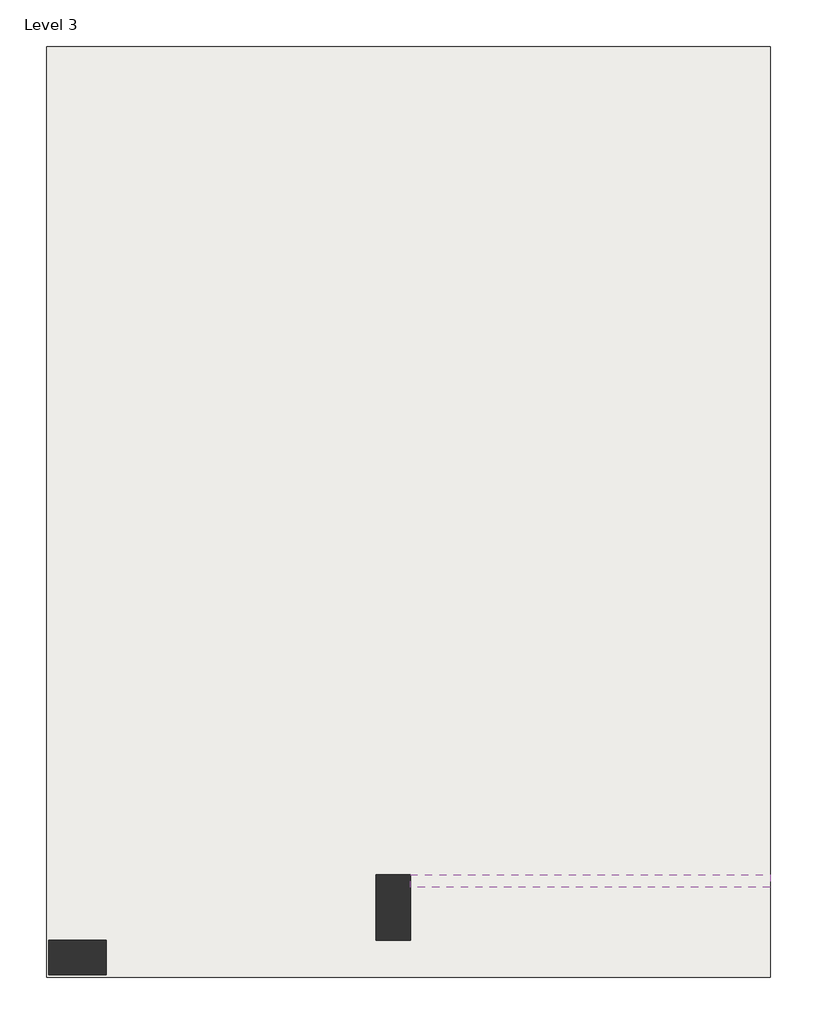
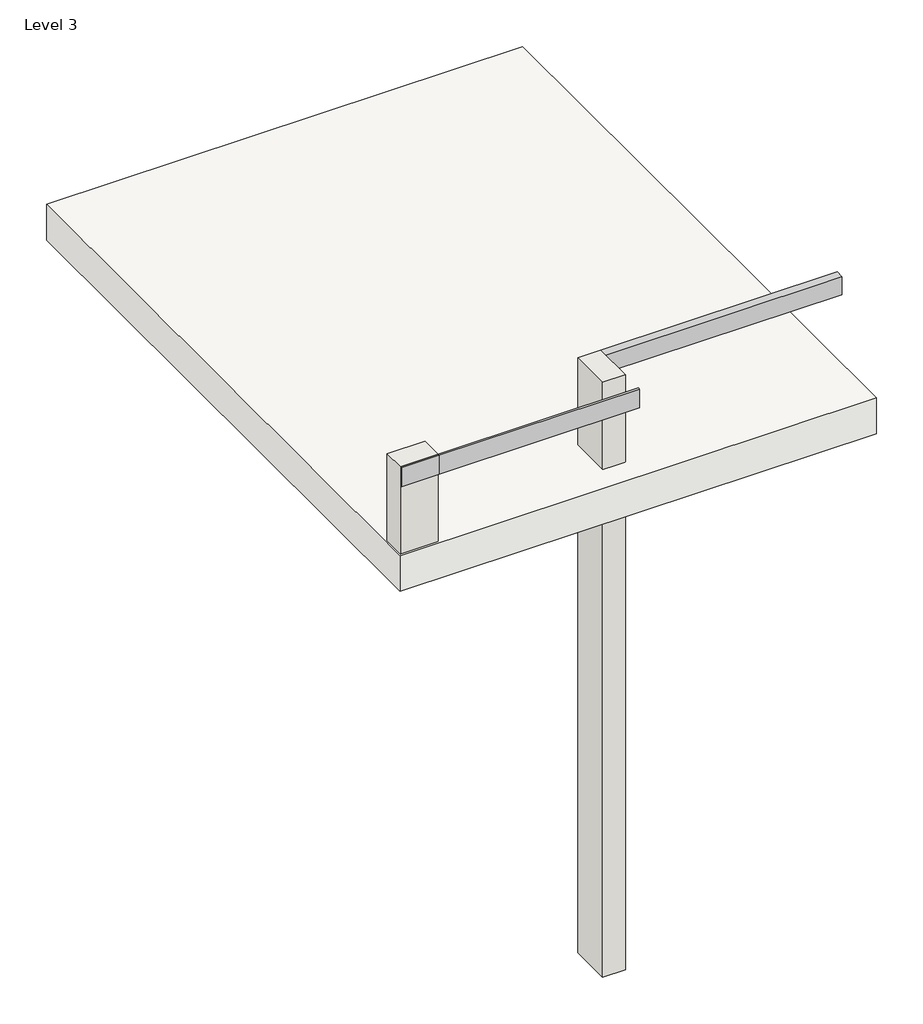
# One storey: 2 walls, 1 proxy, 1 roof.
"""IFC4 building model written with IfcOpenShell, lengths in millimetres."""

from ifc_helpers import new_model, si_unit, frame, origin, place, context, project, spatial, polyline, outline, extrude, faceted_brep, transform, mapped, element, save
from components import generic_models_1_generic_models_1_5385a8bd

model = new_model("IFC4")

# Units and contexts
model_context = context("Model", 3, world=origin())
ifc_project = project(units=[si_unit("LENGTHUNIT", "METRE", prefix="MILLI")], contexts=[model_context])

# Site, building, storey
site = spatial("IfcSite", under=ifc_project)
building = spatial("IfcBuilding", under=site)
storey = spatial("IfcBuildingStorey", under=building, Name="Level 3", Elevation=6705.6)

# Proxy
placement = place(None, origin())
generic_models_1_generic_models_1_shape = generic_models_1_generic_models_1_5385a8bd(model_context)
element("IfcBuildingElementProxy", 1, Name="Generic Models 1 : Generic Models 1", ObjectType="Generic Models 1 : Generic Models 1", at=placement, inside=storey, context=model_context, shape_type="MappedRepresentation", body=[
    mapped(generic_models_1_generic_models_1_shape, transform((0.0, 0.0, 0.0), x_axis=(1.0, 0.0, 0.0), y_axis=(0.0, 1.0, 0.0), z_axis=(0.0, 0.0, 1.0))),
])

# Roof
element("IfcRoof", 2, ObjectType="Generic - 18\"", at=placement, inside=storey, context=model_context, shape_type="SweptSolid", body=[
    extrude(outline(polyline([(-13364.9465329, 11213.7598519), (-6964.1465329, 11213.7598519), (-6964.1465329, 2984.1598519), (-13364.9465329, 2984.1598519), (-13364.9465329, 11213.7598519)])), frame((0.0, 0.0, 6705.6), z_axis=(0.0, 0.0, 1.0), x_axis=(1.0, 0.0, 0.0)), (0.0, 0.0, 1.0), 508.0),
])

# Walls
element("IfcWall", 3, ObjectType="Generic - 12\"", at=placement, inside=storey, context=model_context, shape_type="Brep", body=[
    faceted_brep([(-12837.2306534, 3314.3598519, 6705.6), (-13345.2306534, 3314.3598519, 6705.6), (-13345.2306534, 3314.3598519, 7213.6), (-13345.2306534, 3314.3598519, 8451.8321088), (-12837.2306534, 3314.3598519, 8451.8321088), (-12837.2306534, 3314.3598519, 7213.6), (-12837.2306534, 3009.5598519, 6705.6), (-12837.2306534, 3009.5598519, 8451.8321088), (-13345.2306534, 3009.5598519, 8451.8321088), (-13345.2306534, 3009.5598519, 6705.6)], [[[0, 1, 2, 3, 4, 5]], [[6, 7, 8, 9]], [[1, 0, 6, 9]], [[3, 2, 1, 9, 8]], [[4, 3, 8, 7]], [[0, 5, 4, 7, 6]]]),
])
element("IfcWall", 4, ObjectType="Generic - 12\"", at=placement, inside=storey, context=model_context, shape_type="Brep", body=[
    faceted_brep([(-10144.8306534, 3314.3598519, 0.0), (-10144.8306534, 3890.6797737, 0.0), (-10144.8306534, 3890.6797737, 8451.8321088), (-10144.8306534, 3314.3598519, 8451.8321088), (-10144.8306534, 3314.3598519, 3048.0), (-10449.6306534, 3314.3598519, 0.0), (-10449.6306534, 3314.3598519, 8451.8321088), (-10449.6306534, 3890.6797737, 8451.8321088), (-10449.6306534, 3890.6797737, 8396.4882518), (-10449.6306534, 3890.6797737, 7213.6), (-10449.6306534, 3890.6797737, 0.0)], [[[0, 1, 2, 3, 4]], [[5, 6, 7, 8, 9, 10]], [[1, 0, 5, 10]], [[3, 2, 7, 6]], [[2, 1, 10, 9, 8, 7]], [[0, 4, 3, 6, 5]]]),
])

save(model, "model.ifc")

# Revit data of these elements
# Type "Generic - 18\""
#   Assembly Code = "B1020"
#   Layers, outside or top first: 1' - 8" no material (function 1)
# Type "Generic - 12\""
#   Assembly Code = "B2010"
#   Layers, outside or top first: 1' - 0" no material (function 1)
# Element 1 (IfcBuildingElementProxy, "Generic Models 1 : Generic Models 1")
#   Phase Created = New Construction
# Element 2 (IfcRoof, "Generic - 18\"")
#   built-in parameter 1001705 = 23.6667 (stored number, unit not read)
#   built-in parameter 1001710 = 33615
#   Phase Created = New Construction
#   Materials on its faces: "Default Roof", "Gypsum Wall Board"
# Element 3 (IfcWall, "Generic - 12\"")
#   Top Offset = 0' - 0"
#   Base Offset = 0' - 0"
#   Unconnected Height = 5' - 8.7493"
#   wall height = 5' - 8.7493"
#   Phase Created = New Construction
#   Base Constraint = Level 3
#   Materials on its faces: "Default Wall"
# Element 4 (IfcWall, "Generic - 12\"")
#   built-in parameter 1001111 = -22' - 0"
#   Top Offset = 0' - 0"
#   Base Offset = -22' - 0"
#   Unconnected Height = 27' - 8.7493"
#   wall height = 27' - 8.7493"
#   Phase Created = New Construction
#   Base Constraint = Level 3
#   Materials on its faces: "Default Wall"
# Materials
#   "Default Roof": colour RGB 88 101 114, transparency 0
#   "Gypsum Wall Board": class "Generic", colour RGB 127 127 127, transparency 0, Description = "Gypsum Wall Board", Cost = 0
#   "Default Wall": colour RGB 128 128 128, transparency 0
